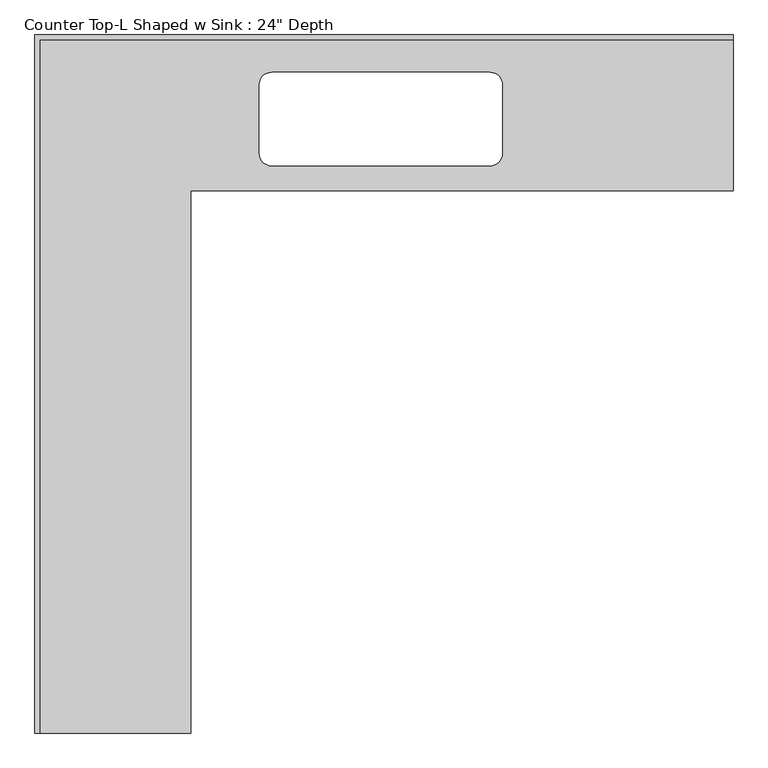
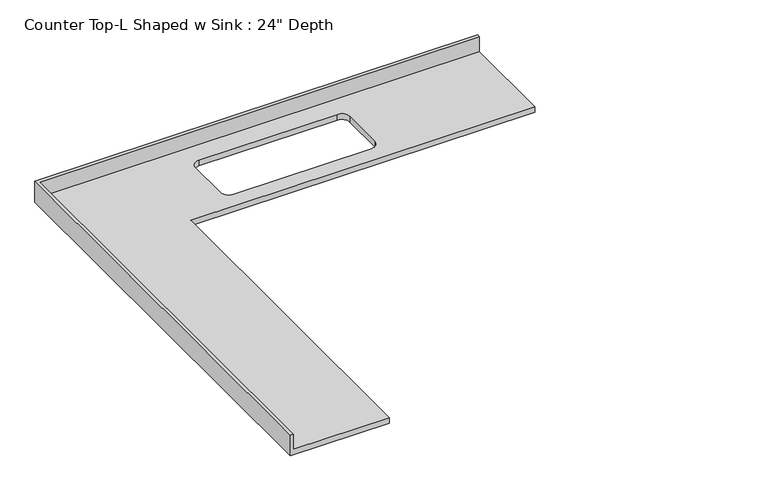
"""IFC4 building model written with IfcOpenShell, lengths in millimetres: furniture geometry."""

from ifc_helpers import new_model, si_unit, frame, origin, place, context, project, spatial, polyline, circle_curve, source, transform, mapped, element, save
from ifc_brep_helpers import plane_surface, revolved_surface, advanced_brep


def furniture_8bbd1b1f(model_context):
    return source(origin(), model_context, "Body", "AdvancedBrep", [
        advanced_brep(
        [(-565.4622951, -2844.8, 914.4), (-565.4622951, -635.0, 914.4), (1644.3377049, -635.0, 914.4), (1644.3377049, -19.05, 914.4), (-1181.4122951, -19.05, 914.4), (-1181.4122951, -2844.8, 914.4), (653.7377049, -152.4, 914.4), (704.5377049, -203.2, 914.4), (704.5377049, -482.6, 914.4), (653.7377049, -533.4, 914.4), (-235.2622951, -533.4, 914.4), (-286.0622951, -482.6, 914.4), (-286.0622951, -203.2, 914.4), (-235.2622951, -152.4, 914.4), (1644.3377049, 0.0, 876.3), (1644.3377049, -635.0, 876.3), (-565.4622951, -635.0, 876.3), (-565.4622951, -2844.8, 876.3), (-1200.4622951, -2844.8, 876.3), (-1200.4622951, 0.0, 876.3), (653.7377049, -152.4, 876.3), (-235.2622951, -152.4, 876.3), (-286.0622951, -203.2, 876.3), (-286.0622951, -482.6, 876.3), (-235.2622951, -533.4, 876.3), (653.7377049, -533.4, 876.3), (704.5377049, -482.6, 876.3), (704.5377049, -203.2, 876.3), (-1200.4622951, 0.0, 1016.0), (1644.3377049, 0.0, 1016.0), (-1200.4622951, -2844.8, 1016.0), (-1181.4122951, -2844.8, 1016.0), (1644.3377049, -19.05, 1016.0), (-1181.4122951, -19.05, 1016.0)],
        [
            (0, 1),
            (1, 2),
            (2, 3),
            (3, 4),
            (4, 5),
            (5, 0),
            (6, 7, circle_curve(frame((653.7377049, -203.2, 914.4), z_axis=(0.0, 0.0, -1.0), x_axis=(1.0, 0.0, 0.0)), 50.8)),
            (7, 8),
            (8, 9, circle_curve(frame((653.7377049, -482.6, 914.4), z_axis=(0.0, 0.0, -1.0), x_axis=(1.0, 0.0, 0.0)), 50.8)),
            (9, 10),
            (10, 11, circle_curve(frame((-235.2622951, -482.6, 914.4), z_axis=(0.0, 0.0, -1.0), x_axis=(1.0, 0.0, 0.0)), 50.8)),
            (11, 12),
            (12, 13, circle_curve(frame((-235.2622951, -203.2, 914.4), z_axis=(0.0, 0.0, -1.0), x_axis=(1.0, 0.0, 0.0)), 50.8)),
            (13, 6),
            (14, 15),
            (15, 16),
            (16, 17),
            (17, 18),
            (18, 19),
            (19, 14),
            (20, 21),
            (21, 22, circle_curve(frame((-235.2622951, -203.2, 876.3), z_axis=(0.0, 0.0, 1.0), x_axis=(1.0, 0.0, 0.0)), 50.8)),
            (22, 23),
            (23, 24, circle_curve(frame((-235.2622951, -482.6, 876.3), z_axis=(0.0, 0.0, 1.0), x_axis=(1.0, 0.0, 0.0)), 50.8)),
            (24, 25),
            (25, 26, circle_curve(frame((653.7377049, -482.6, 876.3), z_axis=(0.0, 0.0, 1.0), x_axis=(1.0, 0.0, 0.0)), 50.8)),
            (26, 27),
            (27, 20, circle_curve(frame((653.7377049, -203.2, 876.3), z_axis=(0.0, 0.0, 1.0), x_axis=(1.0, 0.0, 0.0)), 50.8)),
            (19, 28),
            (28, 29),
            (29, 14),
            (18, 30),
            (30, 28),
            (17, 0),
            (5, 31),
            (31, 30),
            (16, 1),
            (15, 2),
            (29, 32),
            (32, 3),
            (6, 20),
            (27, 7),
            (26, 8),
            (25, 9),
            (24, 10),
            (23, 11),
            (22, 12),
            (21, 13),
            (31, 33),
            (33, 32),
            (33, 4),
        ],
        [
            plane_surface(frame((-1200.4622951, 0.0, 914.4), z_axis=(0.0, 0.0, 1.0), x_axis=(-1.0, 0.0, 0.0))),
            plane_surface(frame((-1200.4622951, 0.0, 876.3), z_axis=(0.0, 0.0, -1.0), x_axis=(1.0, 0.0, 0.0))),
            plane_surface(frame((1644.3377049, 0.0, 914.4), z_axis=(0.0, 1.0, 0.0), x_axis=(0.0, 0.0, -1.0))),
            plane_surface(frame((-1200.4622951, 0.0, 914.4), z_axis=(-1.0, 0.0, 0.0), x_axis=(0.0, 0.0, -1.0))),
            plane_surface(frame((-1200.4622951, -2844.8, 914.4), z_axis=(0.0, -1.0, 0.0), x_axis=(0.0, 0.0, -1.0))),
            plane_surface(frame((-565.4622951, -2844.8, 914.4), z_axis=(1.0, 0.0, 0.0), x_axis=(0.0, 0.0, -1.0))),
            plane_surface(frame((-565.4622951, -635.0, 914.4), z_axis=(0.0, -1.0, 0.0), x_axis=(0.0, 0.0, -1.0))),
            plane_surface(frame((1644.3377049, -635.0, 914.4), z_axis=(1.0, 0.0, 0.0), x_axis=(0.0, 0.0, -1.0))),
            revolved_surface(polyline([(704.5377049, -203.2, 876.3), (704.5377049, -203.2, 914.4)]), (653.7377049, -203.2, 0.0), (0.0, 0.0, -1.0)),
            plane_surface(frame((704.5377049, -203.2, 914.4), z_axis=(-1.0, 0.0, 0.0), x_axis=(0.0, 0.0, -1.0))),
            revolved_surface(polyline([(704.5377049, -482.6, 876.3), (704.5377049, -482.6, 914.4)]), (653.7377049, -482.6, 0.0), (0.0, 0.0, -1.0)),
            plane_surface(frame((653.7377049, -533.4, 914.4), z_axis=(0.0, 1.0, 0.0), x_axis=(0.0, 0.0, -1.0))),
            revolved_surface(polyline([(-184.4622951, -482.6, 876.3), (-184.4622951, -482.6, 914.4)]), (-235.2622951, -482.6, 0.0), (0.0, 0.0, -1.0)),
            plane_surface(frame((-286.0622951, -482.6, 914.4), z_axis=(1.0, 0.0, 0.0), x_axis=(0.0, 0.0, -1.0))),
            revolved_surface(polyline([(-184.4622951, -203.2, 876.3), (-184.4622951, -203.2, 914.4)]), (-235.2622951, -203.2, 0.0), (0.0, 0.0, -1.0)),
            plane_surface(frame((-235.2622951, -152.4, 914.4), z_axis=(0.0, -1.0, 0.0), x_axis=(0.0, 0.0, -1.0))),
            plane_surface(frame((-1200.4622951, 0.0, 1016.0), z_axis=(0.0, 0.0, 1.0), x_axis=(0.0, -1.0, 0.0))),
            plane_surface(frame((-1200.4622951, -19.05, 1016.0), z_axis=(0.0, -1.0, 0.0), x_axis=(0.0, 0.0, -1.0))),
            plane_surface(frame((-1181.4122951, -2844.8, 1016.0), z_axis=(1.0, 0.0, 0.0), x_axis=(0.0, 0.0, -1.0))),
        ],
        [
            (0, [[1, 2, 3, 4, 5, 6], [7, 8, 9, 10, 11, 12, 13, 14]]),
            (1, [[15, 16, 17, 18, 19, 20], [21, 22, 23, 24, 25, 26, 27, 28]]),
            (2, [[-20, 29, 30, 31]]),
            (3, [[-19, 32, 33, -29]]),
            (4, [[-32, -18, 34, -6, 35, 36]]),
            (5, [[-1, -34, -17, 37]]),
            (6, [[-2, -37, -16, 38]]),
            (7, [[-15, -31, 39, 40, -3, -38]]),
            (8, [[-7, 41, -28, 42]]),
            (9, [[-8, -42, -27, 43]]),
            (10, [[-9, -43, -26, 44]]),
            (11, [[-10, -44, -25, 45]]),
            (12, [[-11, -45, -24, 46]]),
            (13, [[-12, -46, -23, 47]]),
            (14, [[-13, -47, -22, 48]]),
            (15, [[-14, -48, -21, -41]]),
            (16, [[-33, -36, 49, 50, -39, -30]]),
            (17, [[-40, -50, 51, -4]]),
            (18, [[-49, -35, -5, -51]]),
        ],
    ),
    ])


if __name__ == "__main__":
    model = new_model("IFC4")
    model_context = context("Model", 3, world=origin())
    ifc_project = project(units=[si_unit("LENGTHUNIT", "METRE", prefix="MILLI")], contexts=[model_context])
    site = spatial("IfcSite", under=ifc_project)
    building = spatial("IfcBuilding", under=site)
    placement = place(None, origin())
    furniture_shape = furniture_8bbd1b1f(model_context)
    element("IfcFurniture", 1, ObjectType="Counter Top-L Shaped w Sink : 24\" Depth", at=placement, inside=building, context=model_context, shape_type="MappedRepresentation", body=[
        mapped(furniture_shape, transform((0.0, 0.0, 0.0), x_axis=(1.0, 0.0, 0.0), y_axis=(0.0, 1.0, 0.0), z_axis=(0.0, 0.0, 1.0))),
    ])
    save(model, "model.ifc")

# Revit data of these elements
# Type "Counter Top-L Shaped w Sink : 24\" Depth"
#   Assembly Code = "C1030400"
#   Counter Thickness = 0' - 1 1/2"
#   Depth = 2' - 1"
#   Height = 3' - 0"
#   Length - Leg 1 [instance default] = 8' - 0"
#   Length - Leg 2 [instance default] = 6' - 0"
#   Sink Location [instance default] = 3' - 0"
#   Sink Location To Wall [instance default] = 0' - 6"
#   Sink Opening Depth [instance default] = 1' - 3"
#   Sink Opening Width [instance default] = 3' - 3"
#   Counter Top Material = none
#   Default Elevation = 0
# Element 1 (IfcFurniture, "Counter Top-L Shaped w Sink : 24\" Depth")
#   Length - Leg 1 = 9' - 4"
#   Length - Leg 2 = 9' - 4"
#   Materials on its faces: "Counter Top"
# Materials
#   "Counter Top": class "Wood", colour RGB 226 177 128, transparency 0
